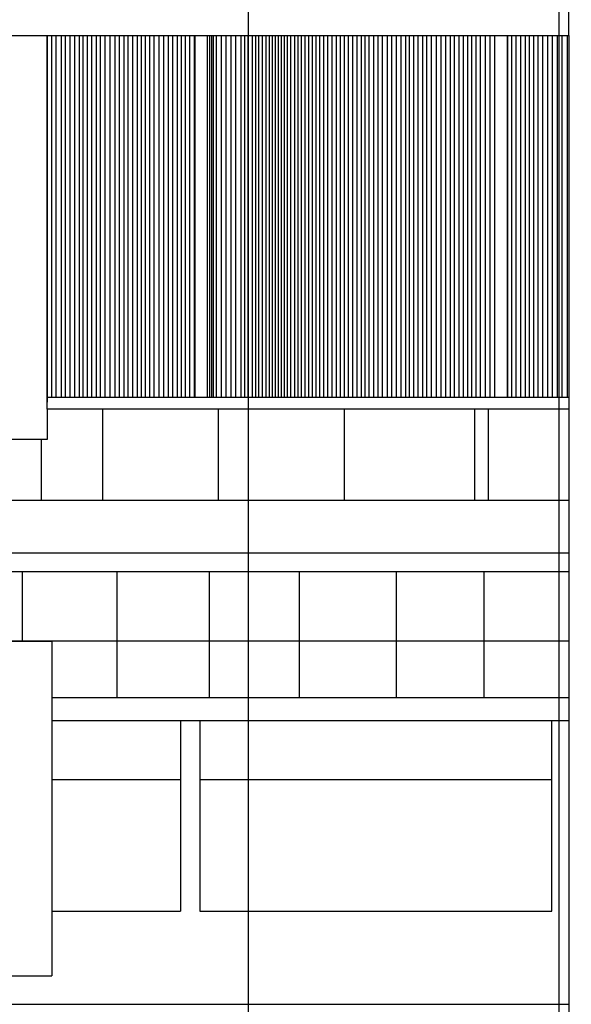
# Model space of a CAD drawing. Units: inches. Extents: x -117 to 121, y -77 to 40.
# Tile 32 of 45: x 47.47 to 57.65, y -7.88 to 10.29. Entities that reach past the tile are written whole.
import ezdxf

# ---------------------------------------------------------------- set-up
doc = ezdxf.new("R2010")
doc.units = ezdxf.units.IN
doc.header["$MEASUREMENT"] = 0
doc.layers.add('A-ANNO-DIMS', color=2, linetype='Continuous', lineweight=18)
doc.layers.add('A-ELEV', color=7, linetype='Continuous', lineweight=25)
doc.styles.get("Standard").update_dxf_attribs({"font": 'arial.ttf'})
doc.dimstyles.get("Standard").update_dxf_attribs({"dimtxt": 0.18, "dimasz": 0.18, "dimexe": 0.18, "dimexo": 0.0625, "dimgap": 0.09, "dimtad": 0, "dimtih": 1, "dimtoh": 1, "dimdec": 4, "dimzin": 0, "dimdsep": 46, "dimtxsty": 'Standard', "dimcen": 0.09, "dimadec": 0, "dimazin": 0, "dimtfac": 1, "dimtdec": 4, "dimtofl": 0, "dimtmove": 0, "dimatfit": 3, "dimfxl": 1, "dimtolj": 1, "dimtzin": 0, "dimarcsym": 0})

# ---------------------------------------------------------------- blocks, each defined once
blk = doc.blocks.new('*D33')
at = {"layer": 'A-ANNO-DIMS', "color": 0, "lineweight": -2, "transparency": 16777216}
for p, q in [((57.433, -43.571), (57.433, 38.61)), ((70.621, -43.571), (70.621, 38.61)), ((57.613, 38.43), (63.572, 38.43)), ((70.441, 38.43), (64.482, 38.43))]:
    blk.add_line(p, q, dxfattribs=at)
at = {"layer": 'A-ANNO-DIMS', "color": 0, "transparency": 16777216}
for points in [[(57.613, 38.46), (57.613, 38.4), (57.433, 38.43)], [(70.441, 38.46), (70.441, 38.4), (70.621, 38.43)]]:
    blk.add_solid(points, dxfattribs=at)
at = {"layer": 'Defpoints', "color": 0, "transparency": 16777216}
for p in [(70.621, 38.43), (57.433, -43.633), (70.621, -43.633)]:
    blk.add_point(p, dxfattribs=at)
at = {"layer": 'A-ANNO-DIMS', "color": 0, "transparency": 16777216, "insert": (64.027, 38.43), "char_height": 0.18, "attachment_point": 5}
blk.add_mtext('\\A1;13.189', dxfattribs=at)
blk = doc.blocks.new('*D53')
at = {"layer": 'A-ANNO-DIMS', "color": 0, "lineweight": -2, "transparency": 16777216}
for p, q in [((27.974, 10.841), (27.974, -77.193)), ((51.69, 10.9), (51.69, -77.193)), ((28.154, -77.013), (39.367, -77.013)), ((51.51, -77.013), (40.297, -77.013))]:
    blk.add_line(p, q, dxfattribs=at)
at = {"layer": 'A-ANNO-DIMS', "color": 0, "transparency": 16777216}
for points in [[(28.154, -76.983), (28.154, -77.043), (27.974, -77.013)], [(51.51, -76.983), (51.51, -77.043), (51.69, -77.013)]]:
    blk.add_solid(points, dxfattribs=at)
at = {"layer": 'Defpoints', "color": 0, "transparency": 16777216}
for p in [(51.69, 10.962), (27.974, 10.903), (51.69, -77.013)]:
    blk.add_point(p, dxfattribs=at)
at = {"layer": 'A-ANNO-DIMS', "color": 0, "transparency": 16777216, "insert": (39.832, -77.013), "char_height": 0.18, "attachment_point": 5}
blk.add_mtext('\\A1;23.716', dxfattribs=at)

msp = doc.modelspace()

# ---------------------------------------------------------------- linework, layer by layer
at = {"layer": 'A-ELEV'}
for p, q in [((57.6104, 9.9998), (57.6104, 10.755)), ((27.8529, 9.9998), (57.6104, 9.9998)), ((47.9835, 3.3186), (47.9835, 9.9998)), ((47.9871, 9.0454), (47.9871, 9.9998)), ((48.0658, 9.0454), (48.0658, 9.9998)), ((48.1476, 9.0454), (48.1476, 9.9998)), ((48.242, 9.0454), (48.242, 9.9998)), ((48.3207, 9.0454), (48.3207, 9.9998)), ((48.4025, 9.0454), (48.4025, 9.9998)), ((48.4904, 9.0454), (48.4904, 9.9998)), ((48.5752, 9.0454), (48.5752, 9.9998)), ((48.6479, 9.0454), (48.6479, 9.9998)), ((48.7236, 9.0454), (48.7236, 9.9998)), ((48.8054, 9.0454), (48.8054, 9.9998)), ((48.8902, 9.0454), (48.8902, 9.9998)), ((48.9659, 9.0454), (48.9659, 9.9998)), ((49.0541, 9.0454), (49.0541, 9.9998)), ((49.142, 9.0454), (49.142, 9.9998)), ((49.2329, 9.0454), (49.2329, 9.9998)), ((49.3146, 9.0454), (49.3146, 9.9998)), ((49.4025, 9.0454), (49.4025, 9.9998)), ((49.4782, 9.0454), (49.4782, 9.9998)), ((49.563, 9.0454), (49.563, 9.9998)), ((49.6448, 9.0454), (49.6448, 9.9998)), ((49.7205, 9.0454), (49.7205, 9.9998)), ((49.7932, 9.0454), (49.7932, 9.9998)), ((49.8756, 9.0454), (49.8756, 9.9998)), ((49.9574, 9.0454), (49.9574, 9.9998)), ((50.0482, 9.0454), (50.0482, 9.9998)), ((50.1331, 9.0454), (50.1331, 9.9998)), ((50.2179, 9.0454), (50.2179, 9.9998)), ((50.3027, 9.0454), (50.3027, 9.9998)), ((50.3845, 9.0454), (50.3845, 9.9998)), ((50.4602, 9.0454), (50.4602, 9.9998)), ((50.5329, 9.0454), (50.5329, 9.9998)), ((50.6147, 9.0454), (50.6147, 9.9998)), ((50.7025, 9.0454), (50.7025, 9.9998)), ((50.7094, 3.3186), (50.7094, 9.9998)), ((50.9388, 9.0454), (50.9388, 9.9998)), ((50.9847, 3.3186), (50.9847, 9.9998)), ((51.0176, 9.0454), (51.0176, 9.9998)), ((51.0529, 3.3186), (51.0529, 9.9998)), ((51.1054, 9.0454), (51.1054, 9.9998)), ((51.1963, 9.0454), (51.1963, 9.9998)), ((51.2841, 9.0454), (51.2841, 9.9998)), ((51.3758, 9.0454), (51.3758, 9.9998)), ((51.4606, 9.0454), (51.4606, 9.9998)), ((51.5636, 9.0454), (51.5636, 9.9998)), ((51.628, 9.0454), (51.628, 9.9998)), ((51.6933, 9.0454), (51.6933, 9.9998)), ((51.7674, 9.0454), (51.7674, 9.9998)), ((51.831, 9.0454), (51.831, 9.9998)), ((51.8885, 9.0454), (51.8885, 9.9998)), ((51.9521, 9.0454), (51.9521, 9.9998)), ((52.0218, 9.0454), (52.0218, 9.9998)), ((52.0824, 9.0454), (52.0824, 9.9998)), ((52.1399, 9.0454), (52.1399, 9.9998)), ((52.1945, 9.0454), (52.1945, 9.9998)), ((52.249, 9.0454), (52.249, 9.9998)), ((52.3035, 9.0454), (52.3035, 9.9998)), ((52.3611, 9.0454), (52.3611, 9.9998)), ((52.4186, 9.0454), (52.4186, 9.9998)), ((52.4796, 9.0454), (52.4796, 9.9998)), ((52.5492, 9.0454), (52.5492, 9.9998)), ((52.6128, 9.0454), (52.6128, 9.9998)), ((52.6734, 9.0454), (52.6734, 9.9998)), ((52.7431, 9.0454), (52.7431, 9.9998)), ((52.8128, 9.0454), (52.8128, 9.9998)), ((52.8794, 9.0454), (52.8794, 9.9998)), ((52.943, 9.0454), (52.943, 9.9998)), ((53.0127, 9.0454), (53.0127, 9.9998)), ((53.0854, 9.0454), (53.0854, 9.9998)), ((53.1581, 9.0454), (53.1581, 9.9998)), ((53.2402, 9.0454), (53.2402, 9.9998)), ((53.319, 9.0454), (53.319, 9.9998)), ((53.3947, 9.0454), (53.3947, 9.9998)), ((53.4674, 9.0454), (53.4674, 9.9998)), ((53.5431, 9.0454), (53.5431, 9.9998)), ((53.6222, 9.0454), (53.6222, 9.9998)), ((53.701, 9.0454), (53.701, 9.9998)), ((53.7797, 9.0454), (53.7797, 9.9998)), ((53.8524, 9.0454), (53.8524, 9.9998)), ((53.9251, 9.0454), (53.9251, 9.9998)), ((54.0099, 9.0454), (54.0099, 9.9998)), ((54.0887, 9.0454), (54.0887, 9.9998)), ((54.1705, 9.0454), (54.1705, 9.9998)), ((54.2648, 9.0454), (54.2648, 9.9998)), ((54.3436, 9.0454), (54.3436, 9.9998)), ((54.4254, 9.0454), (54.4254, 9.9998)), ((54.5132, 9.0454), (54.5132, 9.9998)), ((54.598, 9.0454), (54.598, 9.9998)), ((54.6707, 9.0454), (54.6707, 9.9998)), ((54.7464, 9.0454), (54.7464, 9.9998)), ((54.8282, 9.0454), (54.8282, 9.9998)), ((54.913, 9.0454), (54.913, 9.9998)), ((54.9888, 9.0454), (54.9888, 9.9998)), ((55.077, 9.0454), (55.077, 9.9998)), ((55.1648, 9.0454), (55.1648, 9.9998)), ((55.2557, 9.0454), (55.2557, 9.9998)), ((55.3375, 9.0454), (55.3375, 9.9998)), ((55.4253, 9.0454), (55.4253, 9.9998)), ((55.5011, 9.0454), (55.5011, 9.9998)), ((55.5859, 9.0454), (55.5859, 9.9998)), ((55.6677, 9.0454), (55.6677, 9.9998)), ((55.7434, 9.0454), (55.7434, 9.9998)), ((55.8161, 9.0454), (55.8161, 9.9998)), ((55.8984, 9.0454), (55.8984, 9.9998)), ((55.9802, 9.0454), (55.9802, 9.9998)), ((56.0711, 9.0454), (56.0711, 9.9998)), ((56.1559, 9.0454), (56.1559, 9.9998)), ((56.2407, 9.0454), (56.2407, 9.9998)), ((56.4777, 3.3186), (56.4777, 9.9998)), ((56.4831, 9.0454), (56.4831, 9.9998)), ((56.5558, 9.0454), (56.5558, 9.9998)), ((56.6375, 9.0454), (56.6375, 9.9998)), ((56.7254, 9.0454), (56.7254, 9.9998)), ((56.8102, 9.0454), (56.8102, 9.9998)), ((56.8829, 9.0454), (56.8829, 9.9998)), ((56.9617, 9.0454), (56.9617, 9.9998)), ((57.0404, 9.0454), (57.0404, 9.9998)), ((57.1283, 9.0454), (57.1283, 9.9998)), ((57.2191, 9.0454), (57.2191, 9.9998)), ((57.307, 9.0454), (57.307, 9.9998)), ((57.3987, 9.0454), (57.3987, 9.9998)), ((57.4835, 9.0454), (57.4835, 9.9998)), ((57.5865, 9.0454), (57.5865, 9.9998)), ((57.6104, 9.9998), (57.6104, -2.6527)), ((47.9871, 8.1317), (47.9871, 9.0861)), ((48.0658, 8.1317), (48.0658, 9.0861)), ((48.1476, 8.1317), (48.1476, 9.0861)), ((48.242, 8.1317), (48.242, 9.0861)), ((48.3207, 8.1317), (48.3207, 9.0861)), ((48.4025, 8.1317), (48.4025, 9.0861)), ((48.4904, 8.1317), (48.4904, 9.0861)), ((48.5752, 8.1317), (48.5752, 9.0861)), ((48.6479, 8.1317), (48.6479, 9.0861)), ((48.7236, 8.1317), (48.7236, 9.0861)), ((48.8054, 8.1317), (48.8054, 9.0861)), ((48.8902, 8.1317), (48.8902, 9.0861)), ((48.9659, 8.1317), (48.9659, 9.0861)), ((49.0541, 8.1317), (49.0541, 9.0861)), ((49.142, 8.1317), (49.142, 9.0861)), ((49.2329, 8.1317), (49.2329, 9.0861)), ((49.3146, 8.1317), (49.3146, 9.0861)), ((49.4025, 8.1317), (49.4025, 9.0861)), ((49.4782, 8.1317), (49.4782, 9.0861)), ((49.563, 8.1317), (49.563, 9.0861)), ((49.6448, 8.1317), (49.6448, 9.0861)), ((49.7205, 8.1317), (49.7205, 9.0861)), ((49.7932, 8.1317), (49.7932, 9.0861)), ((49.8756, 8.1317), (49.8756, 9.0861)), ((49.9574, 8.1317), (49.9574, 9.0861)), ((50.0482, 8.1317), (50.0482, 9.0861)), ((50.1331, 8.1317), (50.1331, 9.0861)), ((50.2179, 8.1317), (50.2179, 9.0861)), ((50.3027, 8.1317), (50.3027, 9.0861)), ((50.3845, 8.1317), (50.3845, 9.0861)), ((50.4602, 8.1317), (50.4602, 9.0861)), ((50.5329, 8.1317), (50.5329, 9.0861)), ((50.6147, 8.1317), (50.6147, 9.0861)), ((50.7025, 8.1317), (50.7025, 9.0861)), ((50.9388, 8.1317), (50.9388, 9.0861)), ((51.0176, 8.1317), (51.0176, 9.0861)), ((51.1054, 8.1317), (51.1054, 9.0861)), ((51.1963, 8.1317), (51.1963, 9.0861)), ((51.2841, 8.1317), (51.2841, 9.0861)), ((51.3758, 8.1317), (51.3758, 9.0861)), ((51.4606, 8.1317), (51.4606, 9.0861)), ((51.5636, 8.1317), (51.5636, 9.0861)), ((51.628, 8.1317), (51.628, 9.0861)), ((51.6933, 8.1317), (51.6933, 9.0861)), ((51.7674, 8.1317), (51.7674, 9.0861)), ((51.831, 8.1317), (51.831, 9.0861)), ((51.8885, 8.1317), (51.8885, 9.0861)), ((51.9521, 8.1317), (51.9521, 9.0861)), ((52.0218, 8.1317), (52.0218, 9.0861)), ((52.0824, 8.1317), (52.0824, 9.0861)), ((52.1399, 8.1317), (52.1399, 9.0861)), ((52.1945, 8.1317), (52.1945, 9.0861)), ((52.249, 8.1317), (52.249, 9.0861)), ((52.3035, 8.1317), (52.3035, 9.0861)), ((52.3611, 8.1317), (52.3611, 9.0861)), ((52.4186, 8.1317), (52.4186, 9.0861)), ((52.4796, 8.1317), (52.4796, 9.0861)), ((52.5492, 8.1317), (52.5492, 9.0861)), ((52.6128, 8.1317), (52.6128, 9.0861)), ((52.6734, 8.1317), (52.6734, 9.0861)), ((52.7431, 8.1317), (52.7431, 9.0861)), ((52.8128, 8.1317), (52.8128, 9.0861)), ((52.8794, 8.1317), (52.8794, 9.0861)), ((52.943, 8.1317), (52.943, 9.0861)), ((53.0127, 8.1317), (53.0127, 9.0861)), ((53.0854, 8.1317), (53.0854, 9.0861)), ((53.1581, 8.1317), (53.1581, 9.0861)), ((53.2402, 8.1317), (53.2402, 9.0861)), ((53.319, 8.1317), (53.319, 9.0861)), ((53.3947, 8.1317), (53.3947, 9.0861)), ((53.4674, 8.1317), (53.4674, 9.0861)), ((53.5431, 8.1317), (53.5431, 9.0861)), ((53.6222, 8.1317), (53.6222, 9.0861)), ((53.701, 8.1317), (53.701, 9.0861)), ((53.7797, 8.1317), (53.7797, 9.0861)), ((53.8524, 8.1317), (53.8524, 9.0861)), ((53.9251, 8.1317), (53.9251, 9.0861)), ((54.0099, 8.1317), (54.0099, 9.0861)), ((54.0887, 8.1317), (54.0887, 9.0861)), ((54.1705, 8.1317), (54.1705, 9.0861)), ((54.2648, 8.1317), (54.2648, 9.0861)), ((54.3436, 8.1317), (54.3436, 9.0861)), ((54.4254, 8.1317), (54.4254, 9.0861)), ((54.5132, 8.1317), (54.5132, 9.0861)), ((54.598, 8.1317), (54.598, 9.0861)), ((54.6707, 8.1317), (54.6707, 9.0861)), ((54.7464, 8.1317), (54.7464, 9.0861)), ((54.8282, 8.1317), (54.8282, 9.0861)), ((54.913, 8.1317), (54.913, 9.0861)), ((54.9888, 8.1317), (54.9888, 9.0861)), ((55.077, 8.1317), (55.077, 9.0861)), ((55.1648, 8.1317), (55.1648, 9.0861)), ((55.2557, 8.1317), (55.2557, 9.0861)), ((55.3375, 8.1317), (55.3375, 9.0861)), ((55.4253, 8.1317), (55.4253, 9.0861)), ((55.5011, 8.1317), (55.5011, 9.0861)), ((55.5859, 8.1317), (55.5859, 9.0861)), ((55.6677, 8.1317), (55.6677, 9.0861)), ((55.7434, 8.1317), (55.7434, 9.0861)), ((55.8161, 8.1317), (55.8161, 9.0861)), ((55.8984, 8.1317), (55.8984, 9.0861)), ((55.9802, 8.1317), (55.9802, 9.0861)), ((56.0711, 8.1317), (56.0711, 9.0861)), ((56.1559, 8.1317), (56.1559, 9.0861)), ((56.2407, 8.1317), (56.2407, 9.0861)), ((56.4831, 8.1317), (56.4831, 9.0861)), ((56.5558, 8.1317), (56.5558, 9.0861)), ((56.6375, 8.1317), (56.6375, 9.0861)), ((56.7254, 8.1317), (56.7254, 9.0861)), ((56.8102, 8.1317), (56.8102, 9.0861)), ((56.8829, 8.1317), (56.8829, 9.0861)), ((56.9617, 8.1317), (56.9617, 9.0861)), ((57.0404, 8.1317), (57.0404, 9.0861)), ((57.1283, 8.1317), (57.1283, 9.0861)), ((57.2191, 8.1317), (57.2191, 9.0861)), ((57.307, 8.1317), (57.307, 9.0861)), ((57.3987, 8.1317), (57.3987, 9.0861)), ((57.4835, 8.1317), (57.4835, 9.0861)), ((57.5865, 8.1317), (57.5865, 9.0861)), ((47.9871, 7.1983), (47.9871, 8.1527)), ((48.0658, 7.1983), (48.0658, 8.1527)), ((48.1476, 7.1983), (48.1476, 8.1527)), ((48.242, 7.1983), (48.242, 8.1527)), ((48.3207, 7.1983), (48.3207, 8.1527)), ((48.4025, 7.1983), (48.4025, 8.1527)), ((48.4904, 7.1983), (48.4904, 8.1527)), ((48.5752, 7.1983), (48.5752, 8.1527)), ((48.6479, 7.1983), (48.6479, 8.1527)), ((48.7236, 7.1983), (48.7236, 8.1527)), ((48.8054, 7.1983), (48.8054, 8.1527)), ((48.8902, 7.1983), (48.8902, 8.1527)), ((48.9659, 7.1983), (48.9659, 8.1527)), ((49.0541, 7.1983), (49.0541, 8.1527)), ((49.142, 7.1983), (49.142, 8.1527)), ((49.2329, 7.1983), (49.2329, 8.1527)), ((49.3146, 7.1983), (49.3146, 8.1527)), ((49.4025, 7.1983), (49.4025, 8.1527)), ((49.4782, 7.1983), (49.4782, 8.1527)), ((49.563, 7.1983), (49.563, 8.1527)), ((49.6448, 7.1983), (49.6448, 8.1527)), ((49.7205, 7.1983), (49.7205, 8.1527)), ((49.7932, 7.1983), (49.7932, 8.1527)), ((49.8756, 7.1983), (49.8756, 8.1527)), ((49.9574, 7.1983), (49.9574, 8.1527)), ((50.0482, 7.1983), (50.0482, 8.1527)), ((50.1331, 7.1983), (50.1331, 8.1527)), ((50.2179, 7.1983), (50.2179, 8.1527)), ((50.3027, 7.1983), (50.3027, 8.1527)), ((50.3845, 7.1983), (50.3845, 8.1527)), ((50.4602, 7.1983), (50.4602, 8.1527)), ((50.5329, 7.1983), (50.5329, 8.1527)), ((50.6147, 7.1983), (50.6147, 8.1527)), ((50.7025, 7.1983), (50.7025, 8.1527)), ((50.9388, 7.1983), (50.9388, 8.1527)), ((51.0176, 7.1983), (51.0176, 8.1527)), ((51.1054, 7.1983), (51.1054, 8.1527)), ((51.1963, 7.1983), (51.1963, 8.1527)), ((51.2841, 7.1983), (51.2841, 8.1527)), ((51.3758, 7.1983), (51.3758, 8.1527)), ((51.4606, 7.1983), (51.4606, 8.1527)), ((51.5636, 7.1983), (51.5636, 8.1527)), ((51.628, 7.1983), (51.628, 8.1527)), ((51.6933, 7.1983), (51.6933, 8.1527)), ((51.7674, 7.1983), (51.7674, 8.1527)), ((51.831, 7.1983), (51.831, 8.1527)), ((51.8885, 7.1983), (51.8885, 8.1527)), ((51.9521, 7.1983), (51.9521, 8.1527)), ((52.0218, 7.1983), (52.0218, 8.1527)), ((52.0824, 7.1983), (52.0824, 8.1527)), ((52.1399, 7.1983), (52.1399, 8.1527)), ((52.1945, 7.1983), (52.1945, 8.1527)), ((52.249, 7.1983), (52.249, 8.1527)), ((52.3035, 7.1983), (52.3035, 8.1527)), ((52.3611, 7.1983), (52.3611, 8.1527)), ((52.4186, 7.1983), (52.4186, 8.1527)), ((52.4796, 7.1983), (52.4796, 8.1527)), ((52.5492, 7.1983), (52.5492, 8.1527)), ((52.6128, 7.1983), (52.6128, 8.1527)), ((52.6734, 7.1983), (52.6734, 8.1527)), ((52.7431, 7.1983), (52.7431, 8.1527)), ((52.8128, 7.1983), (52.8128, 8.1527)), ((52.8794, 7.1983), (52.8794, 8.1527)), ((52.943, 7.1983), (52.943, 8.1527)), ((53.0127, 7.1983), (53.0127, 8.1527)), ((53.0854, 7.1983), (53.0854, 8.1527)), ((53.1581, 7.1983), (53.1581, 8.1527)), ((53.2402, 7.1983), (53.2402, 8.1527)), ((53.319, 7.1983), (53.319, 8.1527)), ((53.3947, 7.1983), (53.3947, 8.1527)), ((53.4674, 7.1983), (53.4674, 8.1527)), ((53.5431, 7.1983), (53.5431, 8.1527)), ((53.6222, 7.1983), (53.6222, 8.1527)), ((53.701, 7.1983), (53.701, 8.1527)), ((53.7797, 7.1983), (53.7797, 8.1527)), ((53.8524, 7.1983), (53.8524, 8.1527)), ((53.9251, 7.1983), (53.9251, 8.1527)), ((54.0099, 7.1983), (54.0099, 8.1527)), ((54.0887, 7.1983), (54.0887, 8.1527)), ((54.1705, 7.1983), (54.1705, 8.1527)), ((54.2648, 7.1983), (54.2648, 8.1527)), ((54.3436, 7.1983), (54.3436, 8.1527)), ((54.4254, 7.1983), (54.4254, 8.1527)), ((54.5132, 7.1983), (54.5132, 8.1527)), ((54.598, 7.1983), (54.598, 8.1527)), ((54.6707, 7.1983), (54.6707, 8.1527)), ((54.7464, 7.1983), (54.7464, 8.1527)), ((54.8282, 7.1983), (54.8282, 8.1527)), ((54.913, 7.1983), (54.913, 8.1527)), ((54.9888, 7.1983), (54.9888, 8.1527)), ((55.077, 7.1983), (55.077, 8.1527)), ((55.1648, 7.1983), (55.1648, 8.1527)), ((55.2557, 7.1983), (55.2557, 8.1527)), ((55.3375, 7.1983), (55.3375, 8.1527)), ((55.4253, 7.1983), (55.4253, 8.1527)), ((55.5011, 7.1983), (55.5011, 8.1527)), ((55.5859, 7.1983), (55.5859, 8.1527)), ((55.6677, 7.1983), (55.6677, 8.1527)), ((55.7434, 7.1983), (55.7434, 8.1527)), ((55.8161, 7.1983), (55.8161, 8.1527)), ((55.8984, 7.1983), (55.8984, 8.1527)), ((55.9802, 7.1983), (55.9802, 8.1527)), ((56.0711, 7.1983), (56.0711, 8.1527)), ((56.1559, 7.1983), (56.1559, 8.1527)), ((56.2407, 7.1983), (56.2407, 8.1527)), ((56.4831, 7.1983), (56.4831, 8.1527)), ((56.5558, 7.1983), (56.5558, 8.1527)), ((56.6375, 7.1983), (56.6375, 8.1527)), ((56.7254, 7.1983), (56.7254, 8.1527)), ((56.8102, 7.1983), (56.8102, 8.1527)), ((56.8829, 7.1983), (56.8829, 8.1527)), ((56.9617, 7.1983), (56.9617, 8.1527)), ((57.0404, 7.1983), (57.0404, 8.1527)), ((57.1283, 7.1983), (57.1283, 8.1527)), ((57.2191, 7.1983), (57.2191, 8.1527)), ((57.307, 7.1983), (57.307, 8.1527)), ((57.3987, 7.1983), (57.3987, 8.1527)), ((57.4835, 7.1983), (57.4835, 8.1527)), ((57.5865, 7.1983), (57.5865, 8.1527)), ((47.9871, 6.2641), (47.9871, 7.2185)), ((48.0658, 6.2641), (48.0658, 7.2185)), ((48.1476, 6.2641), (48.1476, 7.2185)), ((48.242, 6.2641), (48.242, 7.2185)), ((48.3207, 6.2641), (48.3207, 7.2185)), ((48.4025, 6.2641), (48.4025, 7.2185)), ((48.4904, 6.2641), (48.4904, 7.2185)), ((48.5752, 6.2641), (48.5752, 7.2185)), ((48.6479, 6.2641), (48.6479, 7.2185)), ((48.7236, 6.2641), (48.7236, 7.2185)), ((48.8054, 6.2641), (48.8054, 7.2185)), ((48.8902, 6.2641), (48.8902, 7.2185)), ((48.9659, 6.2641), (48.9659, 7.2185)), ((49.0541, 6.2641), (49.0541, 7.2185)), ((49.142, 6.2641), (49.142, 7.2185)), ((49.2329, 6.2641), (49.2329, 7.2185)), ((49.3146, 6.2641), (49.3146, 7.2185)), ((49.4025, 6.2641), (49.4025, 7.2185)), ((49.4782, 6.2641), (49.4782, 7.2185)), ((49.563, 6.2641), (49.563, 7.2185)), ((49.6448, 6.2641), (49.6448, 7.2185)), ((49.7205, 6.2641), (49.7205, 7.2185)), ((49.7932, 6.2641), (49.7932, 7.2185)), ((49.8756, 6.2641), (49.8756, 7.2185)), ((49.9574, 6.2641), (49.9574, 7.2185)), ((50.0482, 6.2641), (50.0482, 7.2185)), ((50.1331, 6.2641), (50.1331, 7.2185)), ((50.2179, 6.2641), (50.2179, 7.2185)), ((50.3027, 6.2641), (50.3027, 7.2185)), ((50.3845, 6.2641), (50.3845, 7.2185)), ((50.4602, 6.2641), (50.4602, 7.2185)), ((50.5329, 6.2641), (50.5329, 7.2185)), ((50.6147, 6.2641), (50.6147, 7.2185)), ((50.7025, 6.2641), (50.7025, 7.2185)), ((50.9388, 6.2641), (50.9388, 7.2185)), ((51.0176, 6.2641), (51.0176, 7.2185)), ((51.1054, 6.2641), (51.1054, 7.2185)), ((51.1963, 6.2641), (51.1963, 7.2185)), ((51.2841, 6.2641), (51.2841, 7.2185)), ((51.3758, 6.2641), (51.3758, 7.2185)), ((51.4606, 6.2641), (51.4606, 7.2185)), ((51.5636, 6.2641), (51.5636, 7.2185)), ((51.628, 6.2641), (51.628, 7.2185)), ((51.6933, 6.2641), (51.6933, 7.2185)), ((51.7674, 6.2641), (51.7674, 7.2185)), ((51.831, 6.2641), (51.831, 7.2185)), ((51.8885, 6.2641), (51.8885, 7.2185)), ((51.9521, 6.2641), (51.9521, 7.2185)), ((52.0218, 6.2641), (52.0218, 7.2185)), ((52.0824, 6.2641), (52.0824, 7.2185)), ((52.1399, 6.2641), (52.1399, 7.2185)), ((52.1945, 6.2641), (52.1945, 7.2185)), ((52.249, 6.2641), (52.249, 7.2185)), ((52.3035, 6.2641), (52.3035, 7.2185)), ((52.3611, 6.2641), (52.3611, 7.2185)), ((52.4186, 6.2641), (52.4186, 7.2185)), ((52.4796, 6.2641), (52.4796, 7.2185)), ((52.5492, 6.2641), (52.5492, 7.2185)), ((52.6128, 6.2641), (52.6128, 7.2185)), ((52.6734, 6.2641), (52.6734, 7.2185)), ((52.7431, 6.2641), (52.7431, 7.2185)), ((52.8128, 6.2641), (52.8128, 7.2185)), ((52.8794, 6.2641), (52.8794, 7.2185)), ((52.943, 6.2641), (52.943, 7.2185)), ((53.0127, 6.2641), (53.0127, 7.2185)), ((53.0854, 6.2641), (53.0854, 7.2185)), ((53.1581, 6.2641), (53.1581, 7.2185)), ((53.2402, 6.2641), (53.2402, 7.2185)), ((53.319, 6.2641), (53.319, 7.2185)), ((53.3947, 6.2641), (53.3947, 7.2185)), ((53.4674, 6.2641), (53.4674, 7.2185)), ((53.5431, 6.2641), (53.5431, 7.2185)), ((53.6222, 6.2641), (53.6222, 7.2185)), ((53.701, 6.2641), (53.701, 7.2185)), ((53.7797, 6.2641), (53.7797, 7.2185)), ((53.8524, 6.2641), (53.8524, 7.2185)), ((53.9251, 6.2641), (53.9251, 7.2185)), ((54.0099, 6.2641), (54.0099, 7.2185)), ((54.0887, 6.2641), (54.0887, 7.2185)), ((54.1705, 6.2641), (54.1705, 7.2185)), ((54.2648, 6.2641), (54.2648, 7.2185)), ((54.3436, 6.2641), (54.3436, 7.2185)), ((54.4254, 6.2641), (54.4254, 7.2185)), ((54.5132, 6.2641), (54.5132, 7.2185)), ((54.598, 6.2641), (54.598, 7.2185)), ((54.6707, 6.2641), (54.6707, 7.2185)), ((54.7464, 6.2641), (54.7464, 7.2185)), ((54.8282, 6.2641), (54.8282, 7.2185)), ((54.913, 6.2641), (54.913, 7.2185)), ((54.9888, 6.2641), (54.9888, 7.2185)), ((55.077, 6.2641), (55.077, 7.2185)), ((55.1648, 6.2641), (55.1648, 7.2185)), ((55.2557, 6.2641), (55.2557, 7.2185)), ((55.3375, 6.2641), (55.3375, 7.2185)), ((55.4253, 6.2641), (55.4253, 7.2185)), ((55.5011, 6.2641), (55.5011, 7.2185)), ((55.5859, 6.2641), (55.5859, 7.2185)), ((55.6677, 6.2641), (55.6677, 7.2185)), ((55.7434, 6.2641), (55.7434, 7.2185)), ((55.8161, 6.2641), (55.8161, 7.2185)), ((55.8984, 6.2641), (55.8984, 7.2185)), ((55.9802, 6.2641), (55.9802, 7.2185)), ((56.0711, 6.2641), (56.0711, 7.2185)), ((56.1559, 6.2641), (56.1559, 7.2185)), ((56.2407, 6.2641), (56.2407, 7.2185)), ((56.4831, 6.2641), (56.4831, 7.2185)), ((56.5558, 6.2641), (56.5558, 7.2185)), ((56.6375, 6.2641), (56.6375, 7.2185)), ((56.7254, 6.2641), (56.7254, 7.2185)), ((56.8102, 6.2641), (56.8102, 7.2185)), ((56.8829, 6.2641), (56.8829, 7.2185)), ((56.9617, 6.2641), (56.9617, 7.2185)), ((57.0404, 6.2641), (57.0404, 7.2185)), ((57.1283, 6.2641), (57.1283, 7.2185)), ((57.2191, 6.2641), (57.2191, 7.2185)), ((57.307, 6.2641), (57.307, 7.2185)), ((57.3987, 6.2641), (57.3987, 7.2185)), ((57.4835, 6.2641), (57.4835, 7.2185)), ((57.5865, 6.2641), (57.5865, 7.2185)), ((47.9871, 5.3441), (47.9871, 6.2985)), ((48.0658, 5.3441), (48.0658, 6.2985)), ((48.1476, 5.3441), (48.1476, 6.2985)), ((48.242, 5.3441), (48.242, 6.2985)), ((48.3207, 5.3441), (48.3207, 6.2985)), ((48.4025, 5.3441), (48.4025, 6.2985)), ((48.4904, 5.3441), (48.4904, 6.2985)), ((48.5752, 5.3441), (48.5752, 6.2985)), ((48.6479, 5.3441), (48.6479, 6.2985)), ((48.7236, 5.3441), (48.7236, 6.2985)), ((48.8054, 5.3441), (48.8054, 6.2985)), ((48.8902, 5.3441), (48.8902, 6.2985)), ((48.9659, 5.3441), (48.9659, 6.2985)), ((49.0541, 5.3441), (49.0541, 6.2985)), ((49.142, 5.3441), (49.142, 6.2985)), ((49.2329, 5.3441), (49.2329, 6.2985)), ((49.3146, 5.3441), (49.3146, 6.2985)), ((49.4025, 5.3441), (49.4025, 6.2985)), ((49.4782, 5.3441), (49.4782, 6.2985)), ((49.563, 5.3441), (49.563, 6.2985)), ((49.6448, 5.3441), (49.6448, 6.2985)), ((49.7205, 5.3441), (49.7205, 6.2985)), ((49.7932, 5.3441), (49.7932, 6.2985)), ((49.8756, 5.3441), (49.8756, 6.2985)), ((49.9574, 5.3441), (49.9574, 6.2985)), ((50.0482, 5.3441), (50.0482, 6.2985)), ((50.1331, 5.3441), (50.1331, 6.2985)), ((50.2179, 5.3441), (50.2179, 6.2985)), ((50.3027, 5.3441), (50.3027, 6.2985)), ((50.3845, 5.3441), (50.3845, 6.2985)), ((50.4602, 5.3441), (50.4602, 6.2985)), ((50.5329, 5.3441), (50.5329, 6.2985)), ((50.6147, 5.3441), (50.6147, 6.2985)), ((50.7025, 5.3441), (50.7025, 6.2985)), ((50.9388, 5.3441), (50.9388, 6.2985)), ((51.0176, 5.3441), (51.0176, 6.2985)), ((51.1054, 5.3441), (51.1054, 6.2985)), ((51.1963, 5.3441), (51.1963, 6.2985)), ((51.2841, 5.3441), (51.2841, 6.2985)), ((51.3758, 5.3441), (51.3758, 6.2985)), ((51.4606, 5.3441), (51.4606, 6.2985)), ((51.5636, 5.3441), (51.5636, 6.2985)), ((51.628, 5.3441), (51.628, 6.2985)), ((51.6933, 5.3441), (51.6933, 6.2985)), ((51.7674, 5.3441), (51.7674, 6.2985)), ((51.831, 5.3441), (51.831, 6.2985)), ((51.8885, 5.3441), (51.8885, 6.2985)), ((51.9521, 5.3441), (51.9521, 6.2985)), ((52.0218, 5.3441), (52.0218, 6.2985)), ((52.0824, 5.3441), (52.0824, 6.2985)), ((52.1399, 5.3441), (52.1399, 6.2985)), ((52.1945, 5.3441), (52.1945, 6.2985)), ((52.249, 5.3441), (52.249, 6.2985)), ((52.3035, 5.3441), (52.3035, 6.2985)), ((52.3611, 5.3441), (52.3611, 6.2985)), ((52.4186, 5.3441), (52.4186, 6.2985)), ((52.4796, 5.3441), (52.4796, 6.2985)), ((52.5492, 5.3441), (52.5492, 6.2985)), ((52.6128, 5.3441), (52.6128, 6.2985)), ((52.6734, 5.3441), (52.6734, 6.2985)), ((52.7431, 5.3441), (52.7431, 6.2985)), ((52.8128, 5.3441), (52.8128, 6.2985)), ((52.8794, 5.3441), (52.8794, 6.2985)), ((52.943, 5.3441), (52.943, 6.2985)), ((53.0127, 5.3441), (53.0127, 6.2985)), ((53.0854, 5.3441), (53.0854, 6.2985)), ((53.1581, 5.3441), (53.1581, 6.2985)), ((53.2402, 5.3441), (53.2402, 6.2985)), ((53.319, 5.3441), (53.319, 6.2985)), ((53.3947, 5.3441), (53.3947, 6.2985)), ((53.4674, 5.3441), (53.4674, 6.2985)), ((53.5431, 5.3441), (53.5431, 6.2985)), ((53.6222, 5.3441), (53.6222, 6.2985)), ((53.701, 5.3441), (53.701, 6.2985)), ((53.7797, 5.3441), (53.7797, 6.2985)), ((53.8524, 5.3441), (53.8524, 6.2985)), ((53.9251, 5.3441), (53.9251, 6.2985)), ((54.0099, 5.3441), (54.0099, 6.2985)), ((54.0887, 5.3441), (54.0887, 6.2985)), ((54.1705, 5.3441), (54.1705, 6.2985)), ((54.2648, 5.3441), (54.2648, 6.2985)), ((54.3436, 5.3441), (54.3436, 6.2985)), ((54.4254, 5.3441), (54.4254, 6.2985)), ((54.5132, 5.3441), (54.5132, 6.2985)), ((54.598, 5.3441), (54.598, 6.2985)), ((54.6707, 5.3441), (54.6707, 6.2985)), ((54.7464, 5.3441), (54.7464, 6.2985)), ((54.8282, 5.3441), (54.8282, 6.2985)), ((54.913, 5.3441), (54.913, 6.2985)), ((54.9888, 5.3441), (54.9888, 6.2985)), ((55.077, 5.3441), (55.077, 6.2985)), ((55.1648, 5.3441), (55.1648, 6.2985)), ((55.2557, 5.3441), (55.2557, 6.2985)), ((55.3375, 5.3441), (55.3375, 6.2985)), ((55.4253, 5.3441), (55.4253, 6.2985)), ((55.5011, 5.3441), (55.5011, 6.2985)), ((55.5859, 5.3441), (55.5859, 6.2985)), ((55.6677, 5.3441), (55.6677, 6.2985)), ((55.7434, 5.3441), (55.7434, 6.2985)), ((55.8161, 5.3441), (55.8161, 6.2985)), ((55.8984, 5.3441), (55.8984, 6.2985)), ((55.9802, 5.3441), (55.9802, 6.2985)), ((56.0711, 5.3441), (56.0711, 6.2985)), ((56.1559, 5.3441), (56.1559, 6.2985)), ((56.2407, 5.3441), (56.2407, 6.2985)), ((56.4831, 5.3441), (56.4831, 6.2985)), ((56.5558, 5.3441), (56.5558, 6.2985)), ((56.6375, 5.3441), (56.6375, 6.2985)), ((56.7254, 5.3441), (56.7254, 6.2985)), ((56.8102, 5.3441), (56.8102, 6.2985)), ((56.8829, 5.3441), (56.8829, 6.2985)), ((56.9617, 5.3441), (56.9617, 6.2985)), ((57.0404, 5.3441), (57.0404, 6.2985)), ((57.1283, 5.3441), (57.1283, 6.2985)), ((57.2191, 5.3441), (57.2191, 6.2985)), ((57.307, 5.3441), (57.307, 6.2985)), ((57.3987, 5.3441), (57.3987, 6.2985)), ((57.4835, 5.3441), (57.4835, 6.2985)), ((57.5865, 5.3441), (57.5865, 6.2985)), ((47.9871, 4.4303), (47.9871, 5.3847)), ((48.0658, 4.4303), (48.0658, 5.3847)), ((48.1476, 4.4303), (48.1476, 5.3847)), ((48.242, 4.4303), (48.242, 5.3847)), ((48.3207, 4.4303), (48.3207, 5.3847)), ((48.4025, 4.4303), (48.4025, 5.3847)), ((48.4904, 4.4303), (48.4904, 5.3847)), ((48.5752, 4.4303), (48.5752, 5.3847)), ((48.6479, 4.4303), (48.6479, 5.3847)), ((48.7236, 4.4303), (48.7236, 5.3847)), ((48.8054, 4.4303), (48.8054, 5.3847)), ((48.8902, 4.4303), (48.8902, 5.3847)), ((48.9659, 4.4303), (48.9659, 5.3847)), ((49.0541, 4.4303), (49.0541, 5.3847)), ((49.142, 4.4303), (49.142, 5.3847)), ((49.2329, 4.4303), (49.2329, 5.3847)), ((49.3146, 4.4303), (49.3146, 5.3847)), ((49.4025, 4.4303), (49.4025, 5.3847)), ((49.4782, 4.4303), (49.4782, 5.3847)), ((49.563, 4.4303), (49.563, 5.3847)), ((49.6448, 4.4303), (49.6448, 5.3847)), ((49.7205, 4.4303), (49.7205, 5.3847)), ((49.7932, 4.4303), (49.7932, 5.3847)), ((49.8756, 4.4303), (49.8756, 5.3847)), ((49.9574, 4.4303), (49.9574, 5.3847)), ((50.0482, 4.4303), (50.0482, 5.3847)), ((50.1331, 4.4303), (50.1331, 5.3847)), ((50.2179, 4.4303), (50.2179, 5.3847)), ((50.3027, 4.4303), (50.3027, 5.3847)), ((50.3845, 4.4303), (50.3845, 5.3847)), ((50.4602, 4.4303), (50.4602, 5.3847)), ((50.5329, 4.4303), (50.5329, 5.3847)), ((50.6147, 4.4303), (50.6147, 5.3847)), ((50.7025, 4.4303), (50.7025, 5.3847)), ((50.9388, 4.4303), (50.9388, 5.3847)), ((51.0176, 4.4303), (51.0176, 5.3847)), ((51.1054, 4.4303), (51.1054, 5.3847)), ((51.1963, 4.4303), (51.1963, 5.3847)), ((51.2841, 4.4303), (51.2841, 5.3847)), ((51.3758, 4.4303), (51.3758, 5.3847)), ((51.4606, 4.4303), (51.4606, 5.3847)), ((51.5636, 4.4303), (51.5636, 5.3847)), ((51.628, 4.4303), (51.628, 5.3847)), ((51.6933, 4.4303), (51.6933, 5.3847)), ((51.7674, 4.4303), (51.7674, 5.3847)), ((51.831, 4.4303), (51.831, 5.3847)), ((51.8885, 4.4303), (51.8885, 5.3847)), ((51.9521, 4.4303), (51.9521, 5.3847)), ((52.0218, 4.4303), (52.0218, 5.3847)), ((52.0824, 4.4303), (52.0824, 5.3847)), ((52.1399, 4.4303), (52.1399, 5.3847)), ((52.1945, 4.4303), (52.1945, 5.3847)), ((52.249, 4.4303), (52.249, 5.3847)), ((52.3035, 4.4303), (52.3035, 5.3847)), ((52.3611, 4.4303), (52.3611, 5.3847)), ((52.4186, 4.4303), (52.4186, 5.3847)), ((52.4796, 4.4303), (52.4796, 5.3847)), ((52.5492, 4.4303), (52.5492, 5.3847)), ((52.6128, 4.4303), (52.6128, 5.3847)), ((52.6734, 4.4303), (52.6734, 5.3847)), ((52.7431, 4.4303), (52.7431, 5.3847)), ((52.8128, 4.4303), (52.8128, 5.3847)), ((52.8794, 4.4303), (52.8794, 5.3847)), ((52.943, 4.4303), (52.943, 5.3847)), ((53.0127, 4.4303), (53.0127, 5.3847)), ((53.0854, 4.4303), (53.0854, 5.3847)), ((53.1581, 4.4303), (53.1581, 5.3847)), ((53.2402, 4.4303), (53.2402, 5.3847)), ((53.319, 4.4303), (53.319, 5.3847)), ((53.3947, 4.4303), (53.3947, 5.3847)), ((53.4674, 4.4303), (53.4674, 5.3847)), ((53.5431, 4.4303), (53.5431, 5.3847)), ((53.6222, 4.4303), (53.6222, 5.3847)), ((53.701, 4.4303), (53.701, 5.3847)), ((53.7797, 4.4303), (53.7797, 5.3847)), ((53.8524, 4.4303), (53.8524, 5.3847)), ((53.9251, 4.4303), (53.9251, 5.3847)), ((54.0099, 4.4303), (54.0099, 5.3847)), ((54.0887, 4.4303), (54.0887, 5.3847)), ((54.1705, 4.4303), (54.1705, 5.3847)), ((54.2648, 4.4303), (54.2648, 5.3847)), ((54.3436, 4.4303), (54.3436, 5.3847)), ((54.4254, 4.4303), (54.4254, 5.3847)), ((54.5132, 4.4303), (54.5132, 5.3847)), ((54.598, 4.4303), (54.598, 5.3847)), ((54.6707, 4.4303), (54.6707, 5.3847)), ((54.7464, 4.4303), (54.7464, 5.3847)), ((54.8282, 4.4303), (54.8282, 5.3847)), ((54.913, 4.4303), (54.913, 5.3847)), ((54.9888, 4.4303), (54.9888, 5.3847)), ((55.077, 4.4303), (55.077, 5.3847)), ((55.1648, 4.4303), (55.1648, 5.3847)), ((55.2557, 4.4303), (55.2557, 5.3847)), ((55.3375, 4.4303), (55.3375, 5.3847)), ((55.4253, 4.4303), (55.4253, 5.3847)), ((55.5011, 4.4303), (55.5011, 5.3847)), ((55.5859, 4.4303), (55.5859, 5.3847)), ((55.6677, 4.4303), (55.6677, 5.3847)), ((55.7434, 4.4303), (55.7434, 5.3847)), ((55.8161, 4.4303), (55.8161, 5.3847)), ((55.8984, 4.4303), (55.8984, 5.3847)), ((55.9802, 4.4303), (55.9802, 5.3847)), ((56.0711, 4.4303), (56.0711, 5.3847)), ((56.1559, 4.4303), (56.1559, 5.3847)), ((56.2407, 4.4303), (56.2407, 5.3847)), ((56.4831, 4.4303), (56.4831, 5.3847)), ((56.5558, 4.4303), (56.5558, 5.3847)), ((56.6375, 4.4303), (56.6375, 5.3847)), ((56.7254, 4.4303), (56.7254, 5.3847)), ((56.8102, 4.4303), (56.8102, 5.3847)), ((56.8829, 4.4303), (56.8829, 5.3847)), ((56.9617, 4.4303), (56.9617, 5.3847)), ((57.0404, 4.4303), (57.0404, 5.3847)), ((57.1283, 4.4303), (57.1283, 5.3847)), ((57.2191, 4.4303), (57.2191, 5.3847)), ((57.307, 4.4303), (57.307, 5.3847)), ((57.3987, 4.4303), (57.3987, 5.3847)), ((57.4835, 4.4303), (57.4835, 5.3847)), ((57.5865, 4.4303), (57.5865, 5.3847)), ((47.9871, 4.1736), (47.9871, 5.128)), ((48.0658, 4.1736), (48.0658, 5.128)), ((48.1476, 4.1736), (48.1476, 5.128)), ((48.242, 4.1736), (48.242, 5.128)), ((48.3207, 4.1736), (48.3207, 5.128)), ((48.4025, 4.1736), (48.4025, 5.128)), ((48.4904, 4.1736), (48.4904, 5.128)), ((48.5752, 4.1736), (48.5752, 5.128)), ((48.6479, 4.1736), (48.6479, 5.128)), ((48.7236, 4.1736), (48.7236, 5.128)), ((48.8054, 4.1736), (48.8054, 5.128)), ((48.8902, 4.1736), (48.8902, 5.128)), ((48.9659, 4.1736), (48.9659, 5.128)), ((49.0541, 4.1736), (49.0541, 5.128)), ((49.142, 4.1736), (49.142, 5.128)), ((49.2329, 4.1736), (49.2329, 5.128)), ((49.3146, 4.1736), (49.3146, 5.128)), ((49.4025, 4.1736), (49.4025, 5.128)), ((49.4782, 4.1736), (49.4782, 5.128)), ((49.563, 4.1736), (49.563, 5.128)), ((49.6448, 4.1736), (49.6448, 5.128)), ((49.7205, 4.1736), (49.7205, 5.128)), ((49.7932, 4.1736), (49.7932, 5.128)), ((49.8756, 4.1736), (49.8756, 5.128)), ((49.9574, 4.1736), (49.9574, 5.128)), ((50.0482, 4.1736), (50.0482, 5.128)), ((50.1331, 4.1736), (50.1331, 5.128)), ((50.2179, 4.1736), (50.2179, 5.128)), ((50.3027, 4.1736), (50.3027, 5.128)), ((50.3845, 4.1736), (50.3845, 5.128)), ((50.4602, 4.1736), (50.4602, 5.128)), ((50.5329, 4.1736), (50.5329, 5.128)), ((50.6147, 4.1736), (50.6147, 5.128)), ((50.7025, 4.1736), (50.7025, 5.128)), ((50.9388, 4.1736), (50.9388, 5.128)), ((51.0176, 4.1736), (51.0176, 5.128)), ((51.1054, 4.1736), (51.1054, 5.128)), ((51.1963, 4.1736), (51.1963, 5.128)), ((51.2841, 4.1736), (51.2841, 5.128)), ((51.3758, 4.1736), (51.3758, 5.128)), ((51.4606, 4.1736), (51.4606, 5.128)), ((51.5636, 4.1736), (51.5636, 5.128)), ((51.628, 4.1736), (51.628, 5.128)), ((51.6933, 4.1736), (51.6933, 5.128)), ((51.7674, 4.1736), (51.7674, 5.128)), ((51.831, 4.1736), (51.831, 5.128)), ((51.8885, 4.1736), (51.8885, 5.128)), ((51.9521, 4.1736), (51.9521, 5.128)), ((52.0218, 4.1736), (52.0218, 5.128)), ((52.0824, 4.1736), (52.0824, 5.128)), ((52.1399, 4.1736), (52.1399, 5.128)), ((52.1945, 4.1736), (52.1945, 5.128)), ((52.249, 4.1736), (52.249, 5.128)), ((52.3035, 4.1736), (52.3035, 5.128)), ((52.3611, 4.1736), (52.3611, 5.128)), ((52.4186, 4.1736), (52.4186, 5.128)), ((52.4796, 4.1736), (52.4796, 5.128)), ((52.5492, 4.1736), (52.5492, 5.128)), ((52.6128, 4.1736), (52.6128, 5.128)), ((52.6734, 4.1736), (52.6734, 5.128)), ((52.7431, 4.1736), (52.7431, 5.128)), ((52.8128, 4.1736), (52.8128, 5.128)), ((52.8794, 4.1736), (52.8794, 5.128)), ((52.943, 4.1736), (52.943, 5.128)), ((53.0127, 4.1736), (53.0127, 5.128)), ((53.0854, 4.1736), (53.0854, 5.128)), ((53.1581, 4.1736), (53.1581, 5.128)), ((53.2402, 4.1736), (53.2402, 5.128)), ((53.319, 4.1736), (53.319, 5.128)), ((53.3947, 4.1736), (53.3947, 5.128)), ((53.4674, 4.1736), (53.4674, 5.128)), ((53.5431, 4.1736), (53.5431, 5.128)), ((53.6222, 4.1736), (53.6222, 5.128)), ((53.701, 4.1736), (53.701, 5.128)), ((53.7797, 4.1736), (53.7797, 5.128)), ((53.8524, 4.1736), (53.8524, 5.128)), ((53.9251, 4.1736), (53.9251, 5.128)), ((54.0099, 4.1736), (54.0099, 5.128)), ((54.0887, 4.1736), (54.0887, 5.128)), ((54.1705, 4.1736), (54.1705, 5.128)), ((54.2648, 4.1736), (54.2648, 5.128)), ((54.3436, 4.1736), (54.3436, 5.128)), ((54.4254, 4.1736), (54.4254, 5.128)), ((54.5132, 4.1736), (54.5132, 5.128)), ((54.598, 4.1736), (54.598, 5.128)), ((54.6707, 4.1736), (54.6707, 5.128)), ((54.7464, 4.1736), (54.7464, 5.128)), ((54.8282, 4.1736), (54.8282, 5.128)), ((54.913, 4.1736), (54.913, 5.128)), ((54.9888, 4.1736), (54.9888, 5.128)), ((55.077, 4.1736), (55.077, 5.128)), ((55.1648, 4.1736), (55.1648, 5.128)), ((55.2557, 4.1736), (55.2557, 5.128)), ((55.3375, 4.1736), (55.3375, 5.128)), ((55.4253, 4.1736), (55.4253, 5.128)), ((55.5011, 4.1736), (55.5011, 5.128)), ((55.5859, 4.1736), (55.5859, 5.128)), ((55.6677, 4.1736), (55.6677, 5.128)), ((55.7434, 4.1736), (55.7434, 5.128)), ((55.8161, 4.1736), (55.8161, 5.128)), ((55.8984, 4.1736), (55.8984, 5.128)), ((55.9802, 4.1736), (55.9802, 5.128)), ((56.0711, 4.1736), (56.0711, 5.128)), ((56.1559, 4.1736), (56.1559, 5.128)), ((56.2407, 4.1736), (56.2407, 5.128)), ((56.4831, 4.1736), (56.4831, 5.128)), ((56.5558, 4.1736), (56.5558, 5.128)), ((56.6375, 4.1736), (56.6375, 5.128)), ((56.7254, 4.1736), (56.7254, 5.128)), ((56.8102, 4.1736), (56.8102, 5.128)), ((56.8829, 4.1736), (56.8829, 5.128)), ((56.9617, 4.1736), (56.9617, 5.128)), ((57.0404, 4.1736), (57.0404, 5.128)), ((57.1283, 4.1736), (57.1283, 5.128)), ((57.2191, 4.1736), (57.2191, 5.128)), ((57.307, 4.1736), (57.307, 5.128)), ((57.3987, 4.1736), (57.3987, 5.128)), ((57.4835, 4.1736), (57.4835, 5.128)), ((57.5865, 4.1736), (57.5865, 5.128)), ((47.9871, 3.2323), (47.9871, 4.1867)), ((48.0658, 3.3186), (48.0658, 4.1867)), ((48.1476, 3.3186), (48.1476, 4.1867)), ((48.242, 3.3186), (48.242, 4.1867)), ((48.3207, 3.3186), (48.3207, 4.1867)), ((48.4025, 3.3186), (48.4025, 4.1867)), ((48.4904, 3.3186), (48.4904, 4.1867)), ((48.5752, 3.3186), (48.5752, 4.1867)), ((48.6479, 3.3186), (48.6479, 4.1867)), ((48.7236, 3.3186), (48.7236, 4.1867)), ((48.8054, 3.3186), (48.8054, 4.1867)), ((48.8902, 3.3186), (48.8902, 4.1867)), ((48.9659, 3.3186), (48.9659, 4.1867)), ((49.0541, 3.3186), (49.0541, 4.1867)), ((49.142, 3.3186), (49.142, 4.1867)), ((49.2329, 3.3186), (49.2329, 4.1867)), ((49.3146, 3.3186), (49.3146, 4.1867)), ((49.4025, 3.3186), (49.4025, 4.1867)), ((49.4782, 3.3186), (49.4782, 4.1867)), ((49.563, 3.3186), (49.563, 4.1867)), ((49.6448, 3.3186), (49.6448, 4.1867)), ((49.7205, 3.3186), (49.7205, 4.1867)), ((49.7932, 3.3186), (49.7932, 4.1867)), ((49.8756, 3.3186), (49.8756, 4.1867)), ((49.9574, 3.3186), (49.9574, 4.1867)), ((50.0482, 3.3186), (50.0482, 4.1867)), ((50.1331, 3.3186), (50.1331, 4.1867)), ((50.2179, 3.3186), (50.2179, 4.1867)), ((50.3027, 3.3186), (50.3027, 4.1867)), ((50.3845, 3.3186), (50.3845, 4.1867)), ((50.4602, 3.3186), (50.4602, 4.1867)), ((50.5329, 3.3186), (50.5329, 4.1867)), ((50.6147, 3.3186), (50.6147, 4.1867)), ((50.7025, 3.3186), (50.7025, 4.1867)), ((50.9388, 3.3186), (50.9388, 4.1867)), ((51.0176, 3.3186), (51.0176, 4.1867)), ((51.1054, 3.3186), (51.1054, 4.1867)), ((51.1963, 3.3186), (51.1963, 4.1867)), ((51.2841, 3.3186), (51.2841, 4.1867)), ((51.3758, 3.3186), (51.3758, 4.1867)), ((51.4606, 3.3186), (51.4606, 4.1867)), ((51.5636, 3.3186), (51.5636, 4.1867)), ((51.628, 3.3186), (51.628, 4.1867)), ((51.6933, 3.3186), (51.6933, 4.1867)), ((51.7674, 3.3186), (51.7674, 4.1867)), ((51.831, 3.3186), (51.831, 4.1867)), ((51.8885, 3.3186), (51.8885, 4.1867)), ((51.9521, 3.3186), (51.9521, 4.1867)), ((52.0218, 3.3186), (52.0218, 4.1867)), ((52.0824, 3.3186), (52.0824, 4.1867)), ((52.1399, 3.3186), (52.1399, 4.1867)), ((52.1945, 3.3186), (52.1945, 4.1867)), ((52.249, 3.3186), (52.249, 4.1867)), ((52.3035, 3.3186), (52.3035, 4.1867)), ((52.3611, 3.3186), (52.3611, 4.1867)), ((52.4186, 3.3186), (52.4186, 4.1867)), ((52.4796, 3.3186), (52.4796, 4.1867)), ((52.5492, 3.3186), (52.5492, 4.1867)), ((52.6128, 3.3186), (52.6128, 4.1867)), ((52.6734, 3.3186), (52.6734, 4.1867)), ((52.7431, 3.3186), (52.7431, 4.1867)), ((52.8128, 3.3186), (52.8128, 4.1867)), ((52.8794, 3.3186), (52.8794, 4.1867)), ((52.943, 3.3186), (52.943, 4.1867)), ((53.0127, 3.3186), (53.0127, 4.1867)), ((53.0854, 3.3186), (53.0854, 4.1867)), ((53.1581, 3.3186), (53.1581, 4.1867)), ((53.2402, 3.3186), (53.2402, 4.1867)), ((53.319, 3.3186), (53.319, 4.1867)), ((53.3947, 3.3186), (53.3947, 4.1867)), ((53.4674, 3.3186), (53.4674, 4.1867)), ((53.5431, 3.3186), (53.5431, 4.1867)), ((53.6222, 3.3186), (53.6222, 4.1867)), ((53.701, 3.3186), (53.701, 4.1867)), ((53.7797, 3.3186), (53.7797, 4.1867)), ((53.8524, 3.3186), (53.8524, 4.1867)), ((53.9251, 3.3186), (53.9251, 4.1867)), ((54.0099, 3.3186), (54.0099, 4.1867)), ((54.0887, 3.3186), (54.0887, 4.1867)), ((54.1705, 3.3186), (54.1705, 4.1867)), ((54.2648, 3.3186), (54.2648, 4.1867)), ((54.3436, 3.3186), (54.3436, 4.1867)), ((54.4254, 3.3186), (54.4254, 4.1867)), ((54.5132, 3.3186), (54.5132, 4.1867)), ((54.598, 3.3186), (54.598, 4.1867)), ((54.6707, 3.3186), (54.6707, 4.1867)), ((54.7464, 3.3186), (54.7464, 4.1867)), ((54.8282, 3.3186), (54.8282, 4.1867)), ((54.913, 3.3186), (54.913, 4.1867)), ((54.9888, 3.3186), (54.9888, 4.1867)), ((55.077, 3.3186), (55.077, 4.1867)), ((55.1648, 3.3186), (55.1648, 4.1867)), ((55.2557, 3.3186), (55.2557, 4.1867)), ((55.3375, 3.3186), (55.3375, 4.1867)), ((55.4253, 3.3186), (55.4253, 4.1867)), ((55.5011, 3.3186), (55.5011, 4.1867)), ((55.5859, 3.3186), (55.5859, 4.1867)), ((55.6677, 3.3186), (55.6677, 4.1867)), ((55.7434, 3.3186), (55.7434, 4.1867)), ((55.8161, 3.3186), (55.8161, 4.1867)), ((55.8984, 3.3186), (55.8984, 4.1867)), ((55.9802, 3.3186), (55.9802, 4.1867)), ((56.0711, 3.3186), (56.0711, 4.1867)), ((56.1559, 3.3186), (56.1559, 4.1867)), ((56.2407, 3.3186), (56.2407, 4.1867)), ((56.4831, 3.3186), (56.4831, 4.1867)), ((56.5558, 3.3186), (56.5558, 4.1867)), ((56.6375, 3.3186), (56.6375, 4.1867)), ((56.7254, 3.3186), (56.7254, 4.1867)), ((56.8102, 3.3186), (56.8102, 4.1867)), ((56.8829, 3.3186), (56.8829, 4.1867)), ((56.9617, 3.3186), (56.9617, 4.1867)), ((57.0404, 3.3186), (57.0404, 4.1867)), ((57.1283, 3.3186), (57.1283, 4.1867)), ((57.2191, 3.3186), (57.2191, 4.1867)), ((57.307, 3.3186), (57.307, 4.1867)), ((57.3987, 3.3186), (57.3987, 4.1867)), ((57.4835, 3.3186), (57.4835, 4.1867)), ((57.5865, 3.3186), (57.5865, 4.1867)), ((57.6104, 3.3186), (47.9835, 3.3186)), ((47.9835, 3.1036), (47.9835, 3.3186)), ((57.6104, 3.1036), (47.9835, 3.1036)), ((47.9835, 3.1036), (47.9835, 2.5428)), ((49.0089, 1.4169), (49.0089, 3.1036)), ((51.1452, 1.4169), (51.1452, 3.1036)), ((53.4696, 1.4169), (53.4696, 3.1036)), ((55.8765, 1.4169), (55.8765, 3.1036)), ((56.1238, 1.4169), (56.1238, 3.1036)), ((47.9835, 2.5428), (36.6962, 2.5428)), ((47.8748, 1.4169), (47.8748, 2.5428)), ((57.6104, 1.4169), (44.867, 1.4169)), ((45.6904, 0.4475), (57.6104, 0.4475)), ((45.6904, 0.1069), (57.6104, 0.1069)), ((47.5234, -1.1791), (47.5234, 0.1069)), ((49.2711, -2.224), (49.2711, 0.1069)), ((50.9761, -2.224), (50.9761, 0.1069)), ((52.6386, -2.224), (52.6386, 0.1069)), ((54.4289, -2.224), (54.4289, 0.1069)), ((56.0488, -2.224), (56.0488, 0.1069)), ((41.553, -1.1791), (48.069, -1.1791)), ((57.6104, -1.1791), (45.6904, -1.1791)), ((48.069, -1.1791), (48.069, -5.6546)), ((57.6104, -2.224), (48.069, -2.224)), ((57.6104, -2.6527), (48.069, -2.6527)), ((50.4388, -2.6527), (50.4388, -6.1657)), ((50.7975, -2.6527), (50.7975, -6.1657)), ((57.2965, -6.1657), (57.2965, -2.6527)), ((57.6104, -2.6527), (57.6104, -10.7374)), ((48.069, -3.7354), (50.4388, -3.7354)), ((50.7975, -3.7354), (57.2965, -3.7354)), ((48.069, -5.6546), (48.069, -6.5943)), ((48.069, -6.1657), (50.4388, -6.1657)), ((50.7975, -6.1657), (57.2965, -6.1657)), ((48.069, -6.5943), (48.069, -7.3579)), ((41.553, -7.3579), (48.069, -7.3579)), ((41.553, -7.8846), (57.6104, -7.8846))]:
    msp.add_line(p, q, dxfattribs=at)

# ---------------------------------------------------------------- dimensions: what is measured, and where the dimension line sits
at = {"layer": 'A-ANNO-DIMS'}
for base, p1, p2, picture, middle in [((70.6214, 38.4297), (57.4328, -43.6334), (70.6214, -43.6334), '*D33', (64.0271, 38.4297)), ((51.6901, -77.0135), (27.9744, 10.9032), (51.6901, 10.9623), '*D53', (39.8322, -77.0135))]:
    dim = msp.add_linear_dim(base=base, p1=p1, p2=p2, dimstyle='Standard', override={"dimdec": 3, "dimlfac": 1, "dimrnd": 0, "dimzin": 0, "dimdsep": 46, "dimlunit": 2}, dxfattribs=at)
    dim.commit()
    dim.dimension.update_dxf_attribs({"geometry": picture, "text_midpoint": middle})

doc.saveas('drawing.dxf')
